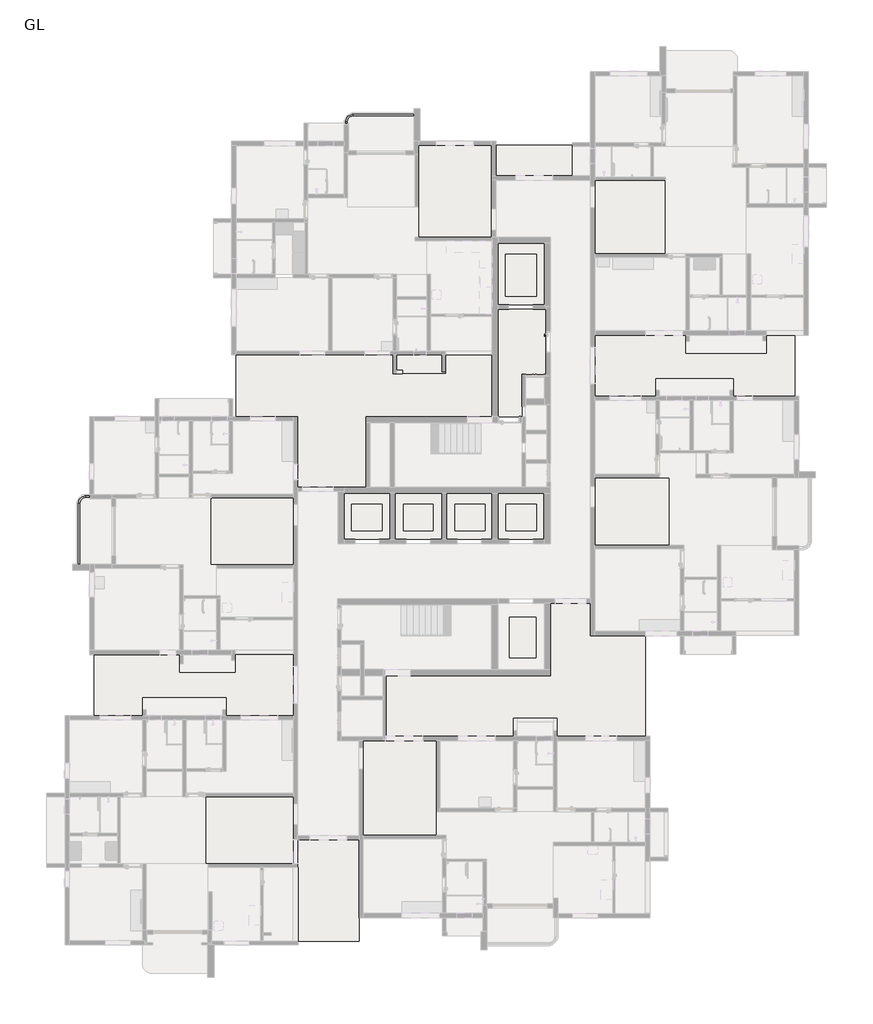
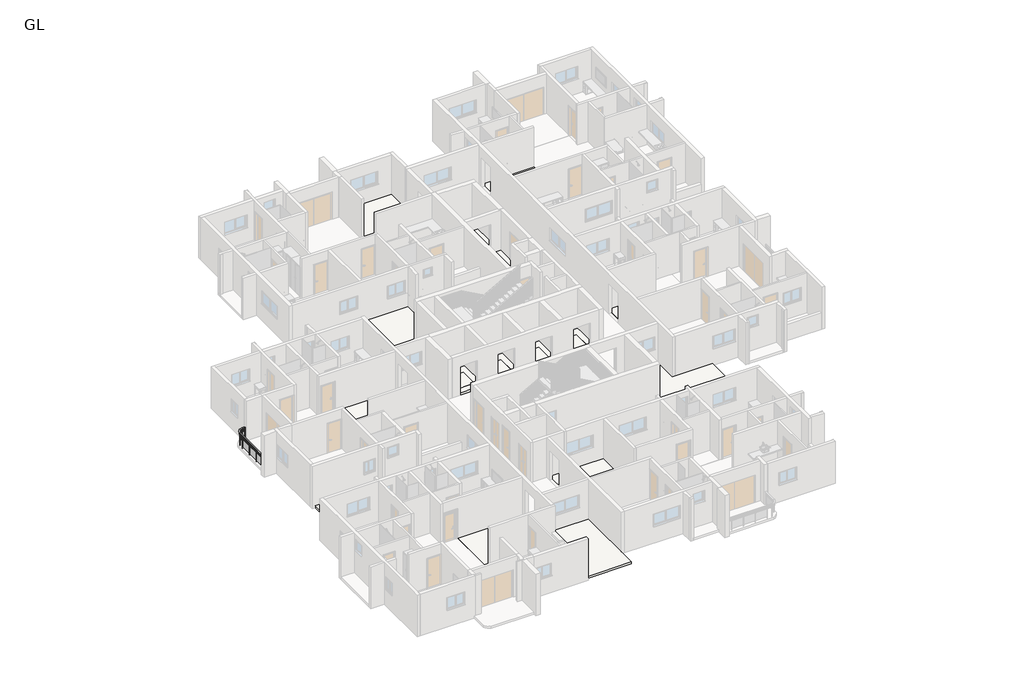
# One storey, part 8 of 14: 6 slabs, 2 railings.
"""IFC4 building model written with IfcOpenShell, lengths in millimetres."""

from ifc_helpers import new_model, si_unit, point, frame, origin, origin_with_axes, place, context, project, spatial, polyline, circle_curve, ellipse_curve, trimmed, outline, extrude, element, save
from ifc_brep_helpers import plane_surface, cylinder_surface, revolved_surface, extruded_surface, advanced_brep

model = new_model("IFC4")

# Units and contexts
model_context = context("Model", 3, world=origin())
ifc_project = project(units=[si_unit("LENGTHUNIT", "METRE", prefix="MILLI")], contexts=[model_context])

# Site, building, storey
site = spatial("IfcSite", under=ifc_project)
building = spatial("IfcBuilding", under=site)
storey = spatial("IfcBuildingStorey", under=building, Name="GL", Elevation=0.0)

# Railings
placement = place(None, origin())
element("IfcRailing", 1, ObjectType="Glass_Panel-Bottom_Fill", at=placement, inside=storey, context=model_context, shape_type="SolidModel", body=[
    advanced_brep(
    [(501.9833716, 97457.1229135, 1049.9616), (501.9833716, 97537.1229135, 1049.9616), (-2551.6680428, 97457.1229135, 1049.9616), (-2551.6680428, 97537.1229135, 1049.9616), (-2919.9542338, 97168.8367225, 1049.9616), (-2839.9542338, 97168.8367225, 1049.9616), (-2839.9542338, 97086.2867225, 1049.9616), (-2919.9542338, 97086.2867225, 1049.9616)],
    [
        (0, 1, ellipse_curve(frame((501.9833716, 97497.1229135, 1049.9616), z_axis=(1.0, 0.0, 0.0), x_axis=(0.0, 1.0, 0.0)), 40.0, 30.0)),
        (1, 0, ellipse_curve(frame((501.9833716, 97497.1229135, 1049.9616), z_axis=(1.0, 0.0, 0.0), x_axis=(0.0, 1.0, 0.0)), 40.0, 30.0)),
        (0, 2),
        (2, 3, ellipse_curve(frame((-2551.6680428, 97497.1229135, 1049.9616), z_axis=(1.0, 0.0, 0.0), x_axis=(0.0, 1.0, 0.0)), 40.0, 30.0)),
        (3, 1),
        (3, 2, ellipse_curve(frame((-2551.6680428, 97497.1229135, 1049.9616), z_axis=(1.0, 0.0, 0.0), x_axis=(0.0, 1.0, 0.0)), 40.0, 30.0)),
        (4, 3, circle_curve(frame((-2551.6680428, 97168.8367225, 1049.9616), z_axis=(0.0, 0.0, -1.0), x_axis=(0.0, 1.0, 0.0)), 368.286191)),
        (2, 5, circle_curve(frame((-2551.6680428, 97168.8367225, 1049.9616), z_axis=(0.0, 0.0, 1.0), x_axis=(0.0, 1.0, 0.0)), 288.286191)),
        (5, 4, ellipse_curve(frame((-2879.9542338, 97168.8367225, 1049.9616), z_axis=(0.0, 1.0, 0.0), x_axis=(-1.0, 0.0, 0.0)), 40.0, 30.0)),
        (4, 5, ellipse_curve(frame((-2879.9542338, 97168.8367225, 1049.9616), z_axis=(0.0, 1.0, 0.0), x_axis=(-1.0, 0.0, 0.0)), 40.0, 30.0)),
        (6, 7, ellipse_curve(frame((-2879.9542338, 97086.2867225, 1049.9616), z_axis=(0.0, -1.0, 0.0), x_axis=(-1.0, 0.0, 0.0)), 40.0, 30.0)),
        (7, 6, ellipse_curve(frame((-2879.9542338, 97086.2867225, 1049.9616), z_axis=(0.0, -1.0, 0.0), x_axis=(-1.0, 0.0, 0.0)), 40.0, 30.0)),
        (5, 6),
        (7, 4),
    ],
    [
        plane_surface(frame((501.9833716, 97497.1229135, 1049.9616), z_axis=(1.0, 0.0, 0.0), x_axis=(0.0, -1.0, 0.0))),
        extruded_surface(trimmed(ellipse_curve(frame((-2551.6680428, 97497.1229135, 1049.9616), z_axis=(1.0, 0.0, 0.0), x_axis=(0.0, 1.0, 0.0)), 40.0, 30.0), [point((-2551.6680428, 97457.1229135, 1049.9616))], [point((-2551.6680428, 97537.1229135, 1049.9616))], True, "CARTESIAN"), (3053.6514144, 0.0, 0.0), 3053.6514144),
        extruded_surface(trimmed(ellipse_curve(frame((-2551.6680428, 97497.1229135, 1049.9616), z_axis=(1.0, 0.0, 0.0), x_axis=(0.0, 1.0, 0.0)), 40.0, 30.0), [point((-2551.6680428, 97537.1229135, 1049.9616))], [point((-2551.6680428, 97457.1229135, 1049.9616))], True, "CARTESIAN"), (3053.6514144, 0.0, 0.0), 3053.6514144),
        revolved_surface(trimmed(ellipse_curve(frame((-2551.6680428, 97497.1229135, 1049.9616), z_axis=(1.0, 0.0, 0.0), x_axis=(0.0, 1.0, 0.0)), 40.0, 30.0), [point((-2551.6680428, 97457.1229135, 1049.9616))], [point((-2551.6680428, 97537.1229135, 1049.9616))], True, "CARTESIAN"), (-2551.6680428, 97168.8367225, 1049.9616), (0.0, 0.0, 1.0)),
        revolved_surface(trimmed(ellipse_curve(frame((-2551.6680428, 97497.1229135, 1049.9616), z_axis=(1.0, 0.0, 0.0), x_axis=(0.0, 1.0, 0.0)), 40.0, 30.0), [point((-2551.6680428, 97537.1229135, 1049.9616))], [point((-2551.6680428, 97457.1229135, 1049.9616))], True, "CARTESIAN"), (-2551.6680428, 97168.8367225, 1049.9616), (0.0, 0.0, 1.0)),
        plane_surface(frame((-2879.9542338, 97086.2867225, 1049.9616), z_axis=(0.0, -1.0, 0.0), x_axis=(0.0, 0.0, -1.0))),
        extruded_surface(trimmed(ellipse_curve(frame((-2879.9542338, 97086.2867225, 1049.9616), z_axis=(0.0, 1.0, 0.0), x_axis=(-1.0, 0.0, 0.0)), 40.0, 30.0), [point((-2839.9542338, 97086.2867225, 1049.9616))], [point((-2919.9542338, 97086.2867225, 1049.9616))], True, "CARTESIAN"), (0.0, 82.55000000000291, 0.0), 82.55000000000291),
        extruded_surface(trimmed(ellipse_curve(frame((-2879.9542338, 97086.2867225, 1049.9616), z_axis=(0.0, 1.0, 0.0), x_axis=(-1.0, 0.0, 0.0)), 40.0, 30.0), [point((-2919.9542338, 97086.2867225, 1049.9616))], [point((-2839.9542338, 97086.2867225, 1049.9616))], True, "CARTESIAN"), (0.0, 82.55000000000291, 0.0), 82.55000000000291),
    ],
    [
        (0, [[1, 2]]),
        (1, [[-1, 3, 4, 5]]),
        (2, [[-2, -5, 6, -3]]),
        (3, [[7, -4, 8, 9]]),
        (4, [[-8, -6, -7, 10]]),
        (5, [[11, 12]]),
        (6, [[-9, 13, -12, 14]]),
        (7, [[-10, -14, -11, -13]]),
    ],
),
    advanced_brep(
    [(501.9833716, 97506.5136787, 949.9616), (501.9833716, 97486.5136787, 949.9616), (501.9833716, 97486.5136787, 929.9616), (501.9833716, 97506.5136787, 929.9616), (-2551.6680428, 97506.5136787, 949.9616), (-2551.6680428, 97486.5136787, 949.9616), (-2551.6680428, 97486.5136787, 929.9616), (-2551.6680428, 97506.5136787, 929.9616), (-2869.344999, 97168.8367225, 949.9616), (-2889.344999, 97168.8367225, 949.9616), (-2869.344999, 97168.8367225, 929.9616), (-2889.344999, 97168.8367225, 929.9616), (-2889.344999, 97086.2867225, 949.9616), (-2889.344999, 97086.2867225, 929.9616), (-2869.344999, 97086.2867225, 929.9616), (-2869.344999, 97086.2867225, 949.9616)],
    [
        (0, 1),
        (1, 2),
        (2, 3),
        (3, 0),
        (0, 4),
        (4, 5),
        (5, 1),
        (5, 6),
        (6, 2),
        (6, 7),
        (7, 3),
        (7, 4),
        (8, 5, circle_curve(frame((-2551.6680428, 97168.8367225, 949.9616), z_axis=(0.0, 0.0, -1.0), x_axis=(0.0, 1.0, 0.0)), 317.6769562)),
        (4, 9, circle_curve(frame((-2551.6680428, 97168.8367225, 949.9616), z_axis=(0.0, 0.0, 1.0), x_axis=(0.0, 1.0, 0.0)), 337.6769562)),
        (9, 8),
        (10, 6, circle_curve(frame((-2551.6680428, 97168.8367225, 929.9616), z_axis=(0.0, 0.0, -1.0), x_axis=(0.0, 1.0, 0.0)), 317.6769562)),
        (8, 10),
        (11, 7, circle_curve(frame((-2551.6680428, 97168.8367225, 929.9616), z_axis=(0.0, 0.0, -1.0), x_axis=(0.0, 1.0, 0.0)), 337.6769562)),
        (10, 11),
        (11, 9),
        (12, 13),
        (13, 14),
        (14, 15),
        (15, 12),
        (9, 12),
        (15, 8),
        (14, 10),
        (13, 11),
    ],
    [
        plane_surface(frame((501.9833716, 97496.5136787, 949.9616), z_axis=(1.0, 0.0, 0.0), x_axis=(0.0, -1.0, 0.0))),
        plane_surface(frame((501.9833716, 97506.5136787, 949.9616), z_axis=(0.0, 0.0, 1.0), x_axis=(-1.0, 0.0, 0.0))),
        plane_surface(frame((501.9833716, 97486.5136787, 949.9616), z_axis=(0.0, -1.0, 0.0), x_axis=(-1.0, 0.0, 0.0))),
        plane_surface(frame((501.9833716, 97486.5136787, 929.9616), z_axis=(0.0, 0.0, -1.0), x_axis=(-1.0, 0.0, 0.0))),
        plane_surface(frame((501.9833716, 97506.5136787, 929.9616), z_axis=(0.0, 1.0, 0.0), x_axis=(-1.0, 0.0, 0.0))),
        plane_surface(frame((-2551.6680428, 97168.8367225, 949.9616), z_axis=(0.0, 0.0, 1.0), x_axis=(0.0, 1.0, 0.0))),
        revolved_surface(polyline([(-2551.6680428, 97486.5136787, 949.9616), (-2551.6680428, 97486.5136787, 929.9616)]), (-2551.6680428, 97168.8367225, 949.9616), (0.0, 0.0, 1.0)),
        plane_surface(frame((-2551.6680428, 97168.8367225, 929.9616), z_axis=(0.0, 0.0, -1.0), x_axis=(0.0, 1.0, 0.0))),
        cylinder_surface(frame((-2551.6680428, 97168.8367225, 949.9616), z_axis=(0.0, 0.0, 1.0), x_axis=(0.0, 1.0, 0.0)), 337.6769562),
        plane_surface(frame((-2879.344999, 97086.2867225, 949.9616), z_axis=(0.0, -1.0, 0.0), x_axis=(0.0, 0.0, -1.0))),
        plane_surface(frame((-2889.344999, 97168.8367225, 949.9616), z_axis=(0.0, 0.0, 1.0), x_axis=(0.0, -1.0, 0.0))),
        plane_surface(frame((-2869.344999, 97168.8367225, 949.9616), z_axis=(1.0, 0.0, 0.0), x_axis=(0.0, -1.0, 0.0))),
        plane_surface(frame((-2869.344999, 97168.8367225, 929.9616), z_axis=(0.0, 0.0, -1.0), x_axis=(0.0, -1.0, 0.0))),
        plane_surface(frame((-2889.344999, 97168.8367225, 929.9616), z_axis=(-1.0, 0.0, 0.0), x_axis=(0.0, -1.0, 0.0))),
    ],
    [
        (0, [[1, 2, 3, 4]]),
        (1, [[-1, 5, 6, 7]]),
        (2, [[-2, -7, 8, 9]]),
        (3, [[-3, -9, 10, 11]]),
        (4, [[-4, -11, 12, -5]]),
        (5, [[13, -6, 14, 15]]),
        (6, [[16, -8, -13, 17]]),
        (7, [[18, -10, -16, 19]]),
        (8, [[-14, -12, -18, 20]]),
        (9, [[21, 22, 23, 24]]),
        (10, [[-15, 25, -24, 26]]),
        (11, [[-17, -26, -23, 27]]),
        (12, [[-19, -27, -22, 28]]),
        (13, [[-20, -28, -21, -25]]),
    ],
),
    advanced_brep(
    [(501.9833716, 97506.5136787, 849.9616), (501.9833716, 97486.5136787, 849.9616), (501.9833716, 97486.5136787, 829.9616), (501.9833716, 97506.5136787, 829.9616), (-2551.6680428, 97506.5136787, 849.9616), (-2551.6680428, 97486.5136787, 849.9616), (-2551.6680428, 97486.5136787, 829.9616), (-2551.6680428, 97506.5136787, 829.9616), (-2869.344999, 97168.8367225, 849.9616), (-2889.344999, 97168.8367225, 849.9616), (-2869.344999, 97168.8367225, 829.9616), (-2889.344999, 97168.8367225, 829.9616), (-2889.344999, 97086.2867225, 849.9616), (-2889.344999, 97086.2867225, 829.9616), (-2869.344999, 97086.2867225, 829.9616), (-2869.344999, 97086.2867225, 849.9616)],
    [
        (0, 1),
        (1, 2),
        (2, 3),
        (3, 0),
        (0, 4),
        (4, 5),
        (5, 1),
        (5, 6),
        (6, 2),
        (6, 7),
        (7, 3),
        (7, 4),
        (8, 5, circle_curve(frame((-2551.6680428, 97168.8367225, 849.9616), z_axis=(0.0, 0.0, -1.0), x_axis=(0.0, 1.0, 0.0)), 317.6769562)),
        (4, 9, circle_curve(frame((-2551.6680428, 97168.8367225, 849.9616), z_axis=(0.0, 0.0, 1.0), x_axis=(0.0, 1.0, 0.0)), 337.6769562)),
        (9, 8),
        (10, 6, circle_curve(frame((-2551.6680428, 97168.8367225, 829.9616), z_axis=(0.0, 0.0, -1.0), x_axis=(0.0, 1.0, 0.0)), 317.6769562)),
        (8, 10),
        (11, 7, circle_curve(frame((-2551.6680428, 97168.8367225, 829.9616), z_axis=(0.0, 0.0, -1.0), x_axis=(0.0, 1.0, 0.0)), 337.6769562)),
        (10, 11),
        (11, 9),
        (12, 13),
        (13, 14),
        (14, 15),
        (15, 12),
        (9, 12),
        (15, 8),
        (14, 10),
        (13, 11),
    ],
    [
        plane_surface(frame((501.9833716, 97496.5136787, 849.9616), z_axis=(1.0, 0.0, 0.0), x_axis=(0.0, -1.0, 0.0))),
        plane_surface(frame((501.9833716, 97506.5136787, 849.9616), z_axis=(0.0, 0.0, 1.0), x_axis=(-1.0, 0.0, 0.0))),
        plane_surface(frame((501.9833716, 97486.5136787, 849.9616), z_axis=(0.0, -1.0, 0.0), x_axis=(-1.0, 0.0, 0.0))),
        plane_surface(frame((501.9833716, 97486.5136787, 829.9616), z_axis=(0.0, 0.0, -1.0), x_axis=(-1.0, 0.0, 0.0))),
        plane_surface(frame((501.9833716, 97506.5136787, 829.9616), z_axis=(0.0, 1.0, 0.0), x_axis=(-1.0, 0.0, 0.0))),
        plane_surface(frame((-2551.6680428, 97168.8367225, 849.9616), z_axis=(0.0, 0.0, 1.0), x_axis=(0.0, 1.0, 0.0))),
        revolved_surface(polyline([(-2551.6680428, 97486.5136787, 849.9616), (-2551.6680428, 97486.5136787, 829.9616)]), (-2551.6680428, 97168.8367225, 849.9616), (0.0, 0.0, 1.0)),
        plane_surface(frame((-2551.6680428, 97168.8367225, 829.9616), z_axis=(0.0, 0.0, -1.0), x_axis=(0.0, 1.0, 0.0))),
        cylinder_surface(frame((-2551.6680428, 97168.8367225, 849.9616), z_axis=(0.0, 0.0, 1.0), x_axis=(0.0, 1.0, 0.0)), 337.6769562),
        plane_surface(frame((-2879.344999, 97086.2867225, 849.9616), z_axis=(0.0, -1.0, 0.0), x_axis=(0.0, 0.0, -1.0))),
        plane_surface(frame((-2889.344999, 97168.8367225, 849.9616), z_axis=(0.0, 0.0, 1.0), x_axis=(0.0, -1.0, 0.0))),
        plane_surface(frame((-2869.344999, 97168.8367225, 849.9616), z_axis=(1.0, 0.0, 0.0), x_axis=(0.0, -1.0, 0.0))),
        plane_surface(frame((-2869.344999, 97168.8367225, 829.9616), z_axis=(0.0, 0.0, -1.0), x_axis=(0.0, -1.0, 0.0))),
        plane_surface(frame((-2889.344999, 97168.8367225, 829.9616), z_axis=(-1.0, 0.0, 0.0), x_axis=(0.0, -1.0, 0.0))),
    ],
    [
        (0, [[1, 2, 3, 4]]),
        (1, [[-1, 5, 6, 7]]),
        (2, [[-2, -7, 8, 9]]),
        (3, [[-3, -9, 10, 11]]),
        (4, [[-4, -11, 12, -5]]),
        (5, [[13, -6, 14, 15]]),
        (6, [[16, -8, -13, 17]]),
        (7, [[18, -10, -16, 19]]),
        (8, [[-14, -12, -18, 20]]),
        (9, [[21, 22, 23, 24]]),
        (10, [[-15, 25, -24, 26]]),
        (11, [[-17, -26, -23, 27]]),
        (12, [[-19, -27, -22, 28]]),
        (13, [[-20, -28, -21, -25]]),
    ],
),
    extrude(outline(polyline([(-2218.8423356, 97471.5136787), (-2230.8423356, 97471.5136787), (-2230.8423356, 97521.5136787), (-2218.8423356, 97521.5136787), (-2218.8423356, 97471.5136787)])), frame((0.0, 0.0, 149.9616), z_axis=(0.0, 0.0, 1.0), x_axis=(1.0, 0.0, 0.0)), (0.0, 0.0, 1.0), 870.0),
    extrude(outline(polyline([(-1424.8423356, 97498.2384888), (-2224.8423356, 97498.2384888), (-2224.8423356, 97503.2384888), (-1424.8423356, 97503.2384888), (-1424.8423356, 97498.2384888)])), frame((0.0, 0.0, 249.9616), z_axis=(0.0, 0.0, 1.0), x_axis=(1.0, 0.0, 0.0)), (0.0, 0.0, 1.0), 580.0),
    extrude(outline(polyline([(-1418.8423356, 97471.5136787), (-1430.8423356, 97471.5136787), (-1430.8423356, 97521.5136787), (-1418.8423356, 97521.5136787), (-1418.8423356, 97471.5136787)])), frame((0.0, 0.0, 149.9616), z_axis=(0.0, 0.0, 1.0), x_axis=(1.0, 0.0, 0.0)), (0.0, 0.0, 1.0), 870.0),
    extrude(outline(polyline([(-624.8423356, 97498.2384888), (-1424.8423356, 97498.2384888), (-1424.8423356, 97503.2384888), (-624.8423356, 97503.2384888), (-624.8423356, 97498.2384888)])), frame((0.0, 0.0, 249.9616), z_axis=(0.0, 0.0, 1.0), x_axis=(1.0, 0.0, 0.0)), (0.0, 0.0, 1.0), 580.0),
    extrude(outline(polyline([(-618.8423356, 97471.5136787), (-630.8423356, 97471.5136787), (-630.8423356, 97521.5136787), (-618.8423356, 97521.5136787), (-618.8423356, 97471.5136787)])), frame((0.0, 0.0, 149.9616), z_axis=(0.0, 0.0, 1.0), x_axis=(1.0, 0.0, 0.0)), (0.0, 0.0, 1.0), 870.0),
    extrude(outline(polyline([(175.1576644, 97498.2384888), (-624.8423356, 97498.2384888), (-624.8423356, 97503.2384888), (175.1576644, 97503.2384888), (175.1576644, 97498.2384888)])), frame((0.0, 0.0, 249.9616), z_axis=(0.0, 0.0, 1.0), x_axis=(1.0, 0.0, 0.0)), (0.0, 0.0, 1.0), 580.0),
    extrude(outline(polyline([(181.1576644, 97471.5136787), (169.1576644, 97471.5136787), (169.1576644, 97521.5136787), (181.1576644, 97521.5136787), (181.1576644, 97471.5136787)])), frame((0.0, 0.0, 149.9616), z_axis=(0.0, 0.0, 1.0), x_axis=(1.0, 0.0, 0.0)), (0.0, 0.0, 1.0), 870.0),
    extrude(outline(polyline([(-2854.344999, 97174.8367225), (-2854.344999, 97162.8367225), (-2904.344999, 97162.8367225), (-2904.344999, 97174.8367225), (-2854.344999, 97174.8367225)])), frame((0.0, 0.0, 149.9616), z_axis=(0.0, 0.0, 1.0), x_axis=(1.0, 0.0, 0.0)), (0.0, 0.0, 1.0), 870.0),
    extrude(outline(polyline([(-2545.6680428, 97471.5136787), (-2557.6680428, 97471.5136787), (-2557.6680428, 97521.5136787), (-2545.6680428, 97521.5136787), (-2545.6680428, 97471.5136787)])), frame((0.0, 0.0, 149.9616), z_axis=(0.0, 0.0, 1.0), x_axis=(1.0, 0.0, 0.0)), (0.0, 0.0, 1.0), 870.0),
    extrude(outline(polyline([(-2854.344999, 97094.2867225), (-2854.344999, 97082.2867225), (-2904.344999, 97082.2867225), (-2904.344999, 97094.2867225), (-2854.344999, 97094.2867225)])), frame((0.0, 0.0, 149.9616), z_axis=(0.0, 0.0, 1.0), x_axis=(1.0, 0.0, 0.0)), (0.0, 0.0, 1.0), 870.0),
    extrude(outline(polyline([(505.9833716, 97471.5136787), (493.9833716, 97471.5136787), (493.9833716, 97521.5136787), (505.9833716, 97521.5136787), (505.9833716, 97471.5136787)])), frame((0.0, 0.0, 149.9616), z_axis=(0.0, 0.0, 1.0), x_axis=(1.0, 0.0, 0.0)), (0.0, 0.0, 1.0), 870.0),
])
element("IfcRailing", 2, ObjectType="Glass_Panel-Bottom_Fill", at=placement, inside=storey, context=model_context, shape_type="SolidModel", body=[
    advanced_brep(
    [(-16238.3038997, 75105.5827724, 1049.9616), (-16158.3038997, 75105.5827724, 1049.9616), (-16238.3038997, 78153.5827724, 1049.9616), (-16158.3038997, 78153.5827724, 1049.9616), (-15865.7412071, 78446.145465, 1049.9616), (-15865.7412071, 78526.145465, 1049.9616), (-15656.6231346, 78526.145465, 1049.9616), (-15656.6231346, 78446.145465, 1049.9616)],
    [
        (0, 1, ellipse_curve(frame((-16198.3038997, 75105.5827724, 1049.9616), z_axis=(0.0, -1.0, 0.0), x_axis=(1.0, 0.0, 0.0)), 40.0, 30.0)),
        (1, 0, ellipse_curve(frame((-16198.3038997, 75105.5827724, 1049.9616), z_axis=(0.0, -1.0, 0.0), x_axis=(1.0, 0.0, 0.0)), 40.0, 30.0)),
        (0, 2),
        (2, 3, ellipse_curve(frame((-16198.3038997, 78153.5827724, 1049.9616), z_axis=(0.0, -1.0, 0.0), x_axis=(1.0, 0.0, 0.0)), 40.0, 30.0)),
        (3, 1),
        (3, 2, ellipse_curve(frame((-16198.3038997, 78153.5827724, 1049.9616), z_axis=(0.0, -1.0, 0.0), x_axis=(1.0, 0.0, 0.0)), 40.0, 30.0)),
        (4, 3, circle_curve(frame((-15865.7412071, 78153.5827724, 1049.9616), z_axis=(0.0, 0.0, 1.0), x_axis=(-1.0, 0.0, 0.0)), 292.5626927)),
        (2, 5, circle_curve(frame((-15865.7412071, 78153.5827724, 1049.9616), z_axis=(0.0, 0.0, -1.0), x_axis=(-1.0, 0.0, 0.0)), 372.5626927)),
        (5, 4, ellipse_curve(frame((-15865.7412071, 78486.145465, 1049.9616), z_axis=(-1.0, 0.0, 0.0), x_axis=(0.0, -1.0, 0.0)), 40.0, 30.0)),
        (4, 5, ellipse_curve(frame((-15865.7412071, 78486.145465, 1049.9616), z_axis=(-1.0, 0.0, 0.0), x_axis=(0.0, -1.0, 0.0)), 40.0, 30.0)),
        (6, 7, ellipse_curve(frame((-15656.6231346, 78486.145465, 1049.9616), z_axis=(1.0, 0.0, 0.0), x_axis=(0.0, -1.0, 0.0)), 40.0, 30.0)),
        (7, 6, ellipse_curve(frame((-15656.6231346, 78486.145465, 1049.9616), z_axis=(1.0, 0.0, 0.0), x_axis=(0.0, -1.0, 0.0)), 40.0, 30.0)),
        (5, 6),
        (7, 4),
    ],
    [
        plane_surface(frame((-16198.3038997, 75105.5827724, 1049.9616), z_axis=(0.0, -1.0, 0.0), x_axis=(0.0, 0.0, 1.0))),
        extruded_surface(trimmed(ellipse_curve(frame((-16198.3038997, 78153.5827724, 1049.9616), z_axis=(0.0, -1.0, 0.0), x_axis=(1.0, 0.0, 0.0)), 40.0, 30.0), [point((-16238.3038997, 78153.5827724, 1049.9616))], [point((-16158.3038997, 78153.5827724, 1049.9616))], True, "CARTESIAN"), (0.0, -3048.0, 0.0), 3048.0),
        extruded_surface(trimmed(ellipse_curve(frame((-16198.3038997, 78153.5827724, 1049.9616), z_axis=(0.0, -1.0, 0.0), x_axis=(1.0, 0.0, 0.0)), 40.0, 30.0), [point((-16158.3038997, 78153.5827724, 1049.9616))], [point((-16238.3038997, 78153.5827724, 1049.9616))], True, "CARTESIAN"), (0.0, -3048.0, 0.0), 3048.0),
        revolved_surface(trimmed(ellipse_curve(frame((-16198.3038997, 78153.5827724, 1049.9616), z_axis=(0.0, -1.0, 0.0), x_axis=(1.0, 0.0, 0.0)), 40.0, 30.0), [point((-16238.3038997, 78153.5827724, 1049.9616))], [point((-16158.3038997, 78153.5827724, 1049.9616))], True, "CARTESIAN"), (-15865.7412071, 78153.5827724, 1049.9616), (0.0, 0.0, -1.0)),
        revolved_surface(trimmed(ellipse_curve(frame((-16198.3038997, 78153.5827724, 1049.9616), z_axis=(0.0, -1.0, 0.0), x_axis=(1.0, 0.0, 0.0)), 40.0, 30.0), [point((-16158.3038997, 78153.5827724, 1049.9616))], [point((-16238.3038997, 78153.5827724, 1049.9616))], True, "CARTESIAN"), (-15865.7412071, 78153.5827724, 1049.9616), (0.0, 0.0, -1.0)),
        plane_surface(frame((-15656.6231346, 78486.145465, 1049.9616), z_axis=(1.0, 0.0, 0.0), x_axis=(0.0, 1.0, 0.0))),
        extruded_surface(trimmed(ellipse_curve(frame((-15656.6231346, 78486.145465, 1049.9616), z_axis=(-1.0, 0.0, 0.0), x_axis=(0.0, -1.0, 0.0)), 40.0, 30.0), [point((-15656.6231346, 78526.145465, 1049.9616))], [point((-15656.6231346, 78446.145465, 1049.9616))], True, "CARTESIAN"), (-209.11807249999947, 0.0, 0.0), 209.11807249999947),
        extruded_surface(trimmed(ellipse_curve(frame((-15656.6231346, 78486.145465, 1049.9616), z_axis=(-1.0, 0.0, 0.0), x_axis=(0.0, -1.0, 0.0)), 40.0, 30.0), [point((-15656.6231346, 78446.145465, 1049.9616))], [point((-15656.6231346, 78526.145465, 1049.9616))], True, "CARTESIAN"), (-209.11807249999947, 0.0, 0.0), 209.11807249999947),
    ],
    [
        (0, [[1, 2]]),
        (1, [[-1, 3, 4, 5]]),
        (2, [[-2, -5, 6, -3]]),
        (3, [[7, -4, 8, 9]]),
        (4, [[-8, -6, -7, 10]]),
        (5, [[11, 12]]),
        (6, [[-9, 13, -12, 14]]),
        (7, [[-10, -14, -11, -13]]),
    ],
),
    advanced_brep(
    [(-16188.9131346, 75105.5827724, 949.9616), (-16208.9131346, 75105.5827724, 949.9616), (-16208.9131346, 75105.5827724, 929.9616), (-16188.9131346, 75105.5827724, 929.9616), (-16188.9131346, 78153.5827724, 949.9616), (-16208.9131346, 78153.5827724, 949.9616), (-16208.9131346, 78153.5827724, 929.9616), (-16188.9131346, 78153.5827724, 929.9616), (-15865.7412071, 78496.7546999, 949.9616), (-15865.7412071, 78476.7546999, 949.9616), (-15865.7412071, 78496.7546999, 929.9616), (-15865.7412071, 78476.7546999, 929.9616), (-15656.6231346, 78476.7546999, 949.9616), (-15656.6231346, 78476.7546999, 929.9616), (-15656.6231346, 78496.7546999, 929.9616), (-15656.6231346, 78496.7546999, 949.9616)],
    [
        (0, 1),
        (1, 2),
        (2, 3),
        (3, 0),
        (0, 4),
        (4, 5),
        (5, 1),
        (5, 6),
        (6, 2),
        (6, 7),
        (7, 3),
        (7, 4),
        (8, 5, circle_curve(frame((-15865.7412071, 78153.5827724, 949.9616), z_axis=(0.0, 0.0, 1.0), x_axis=(-1.0, 0.0, 0.0)), 343.1719275)),
        (4, 9, circle_curve(frame((-15865.7412071, 78153.5827724, 949.9616), z_axis=(0.0, 0.0, -1.0), x_axis=(-1.0, 0.0, 0.0)), 323.1719275)),
        (9, 8),
        (10, 6, circle_curve(frame((-15865.7412071, 78153.5827724, 929.9616), z_axis=(0.0, 0.0, 1.0), x_axis=(-1.0, 0.0, 0.0)), 343.1719275)),
        (8, 10),
        (11, 7, circle_curve(frame((-15865.7412071, 78153.5827724, 929.9616), z_axis=(0.0, 0.0, 1.0), x_axis=(-1.0, 0.0, 0.0)), 323.1719275)),
        (10, 11),
        (11, 9),
        (12, 13),
        (13, 14),
        (14, 15),
        (15, 12),
        (9, 12),
        (15, 8),
        (14, 10),
        (13, 11),
    ],
    [
        plane_surface(frame((-16198.9131346, 75105.5827724, 949.9616), z_axis=(0.0, -1.0, 0.0), x_axis=(0.0, 0.0, 1.0))),
        plane_surface(frame((-16188.9131346, 75105.5827724, 949.9616), z_axis=(0.0, 0.0, 1.0), x_axis=(0.0, 1.0, 0.0))),
        plane_surface(frame((-16208.9131346, 75105.5827724, 949.9616), z_axis=(-1.0, 0.0, 0.0), x_axis=(0.0, 1.0, 0.0))),
        plane_surface(frame((-16208.9131346, 75105.5827724, 929.9616), z_axis=(0.0, 0.0, -1.0), x_axis=(0.0, 1.0, 0.0))),
        plane_surface(frame((-16188.9131346, 75105.5827724, 929.9616), z_axis=(1.0, 0.0, 0.0), x_axis=(0.0, 1.0, 0.0))),
        plane_surface(frame((-15865.7412071, 78153.5827724, 949.9616), z_axis=(0.0, 0.0, 1.0), x_axis=(-1.0, 0.0, 0.0))),
        cylinder_surface(frame((-15865.7412071, 78153.5827724, 949.9616), z_axis=(0.0, 0.0, -1.0), x_axis=(-1.0, 0.0, 0.0)), 343.1719275),
        plane_surface(frame((-15865.7412071, 78153.5827724, 929.9616), z_axis=(0.0, 0.0, -1.0), x_axis=(-1.0, 0.0, 0.0))),
        revolved_surface(polyline([(-16188.9131346, 78153.5827724, 929.9616), (-16188.9131346, 78153.5827724, 949.9616)]), (-15865.7412071, 78153.5827724, 949.9616), (0.0, 0.0, -1.0)),
        plane_surface(frame((-15656.6231346, 78486.7546999, 949.9616), z_axis=(1.0, 0.0, 0.0), x_axis=(0.0, 1.0, 0.0))),
        plane_surface(frame((-15865.7412071, 78476.7546999, 949.9616), z_axis=(0.0, 0.0, 1.0), x_axis=(1.0, 0.0, 0.0))),
        plane_surface(frame((-15865.7412071, 78496.7546999, 949.9616), z_axis=(0.0, 1.0, 0.0), x_axis=(1.0, 0.0, 0.0))),
        plane_surface(frame((-15865.7412071, 78496.7546999, 929.9616), z_axis=(0.0, 0.0, -1.0), x_axis=(1.0, 0.0, 0.0))),
        plane_surface(frame((-15865.7412071, 78476.7546999, 929.9616), z_axis=(0.0, -1.0, 0.0), x_axis=(1.0, 0.0, 0.0))),
    ],
    [
        (0, [[1, 2, 3, 4]]),
        (1, [[-1, 5, 6, 7]]),
        (2, [[-2, -7, 8, 9]]),
        (3, [[-3, -9, 10, 11]]),
        (4, [[-4, -11, 12, -5]]),
        (5, [[13, -6, 14, 15]]),
        (6, [[16, -8, -13, 17]]),
        (7, [[18, -10, -16, 19]]),
        (8, [[-14, -12, -18, 20]]),
        (9, [[21, 22, 23, 24]]),
        (10, [[-15, 25, -24, 26]]),
        (11, [[-17, -26, -23, 27]]),
        (12, [[-19, -27, -22, 28]]),
        (13, [[-20, -28, -21, -25]]),
    ],
),
    advanced_brep(
    [(-16188.9131346, 75105.5827724, 849.9616), (-16208.9131346, 75105.5827724, 849.9616), (-16208.9131346, 75105.5827724, 829.9616), (-16188.9131346, 75105.5827724, 829.9616), (-16188.9131346, 78153.5827724, 849.9616), (-16208.9131346, 78153.5827724, 849.9616), (-16208.9131346, 78153.5827724, 829.9616), (-16188.9131346, 78153.5827724, 829.9616), (-15865.7412071, 78496.7546999, 849.9616), (-15865.7412071, 78476.7546999, 849.9616), (-15865.7412071, 78496.7546999, 829.9616), (-15865.7412071, 78476.7546999, 829.9616), (-15656.6231346, 78476.7546999, 849.9616), (-15656.6231346, 78476.7546999, 829.9616), (-15656.6231346, 78496.7546999, 829.9616), (-15656.6231346, 78496.7546999, 849.9616)],
    [
        (0, 1),
        (1, 2),
        (2, 3),
        (3, 0),
        (0, 4),
        (4, 5),
        (5, 1),
        (5, 6),
        (6, 2),
        (6, 7),
        (7, 3),
        (7, 4),
        (8, 5, circle_curve(frame((-15865.7412071, 78153.5827724, 849.9616), z_axis=(0.0, 0.0, 1.0), x_axis=(-1.0, 0.0, 0.0)), 343.1719275)),
        (4, 9, circle_curve(frame((-15865.7412071, 78153.5827724, 849.9616), z_axis=(0.0, 0.0, -1.0), x_axis=(-1.0, 0.0, 0.0)), 323.1719275)),
        (9, 8),
        (10, 6, circle_curve(frame((-15865.7412071, 78153.5827724, 829.9616), z_axis=(0.0, 0.0, 1.0), x_axis=(-1.0, 0.0, 0.0)), 343.1719275)),
        (8, 10),
        (11, 7, circle_curve(frame((-15865.7412071, 78153.5827724, 829.9616), z_axis=(0.0, 0.0, 1.0), x_axis=(-1.0, 0.0, 0.0)), 323.1719275)),
        (10, 11),
        (11, 9),
        (12, 13),
        (13, 14),
        (14, 15),
        (15, 12),
        (9, 12),
        (15, 8),
        (14, 10),
        (13, 11),
    ],
    [
        plane_surface(frame((-16198.9131346, 75105.5827724, 849.9616), z_axis=(0.0, -1.0, 0.0), x_axis=(0.0, 0.0, 1.0))),
        plane_surface(frame((-16188.9131346, 75105.5827724, 849.9616), z_axis=(0.0, 0.0, 1.0), x_axis=(0.0, 1.0, 0.0))),
        plane_surface(frame((-16208.9131346, 75105.5827724, 849.9616), z_axis=(-1.0, 0.0, 0.0), x_axis=(0.0, 1.0, 0.0))),
        plane_surface(frame((-16208.9131346, 75105.5827724, 829.9616), z_axis=(0.0, 0.0, -1.0), x_axis=(0.0, 1.0, 0.0))),
        plane_surface(frame((-16188.9131346, 75105.5827724, 829.9616), z_axis=(1.0, 0.0, 0.0), x_axis=(0.0, 1.0, 0.0))),
        plane_surface(frame((-15865.7412071, 78153.5827724, 849.9616), z_axis=(0.0, 0.0, 1.0), x_axis=(-1.0, 0.0, 0.0))),
        cylinder_surface(frame((-15865.7412071, 78153.5827724, 849.9616), z_axis=(0.0, 0.0, -1.0), x_axis=(-1.0, 0.0, 0.0)), 343.1719275),
        plane_surface(frame((-15865.7412071, 78153.5827724, 829.9616), z_axis=(0.0, 0.0, -1.0), x_axis=(-1.0, 0.0, 0.0))),
        revolved_surface(polyline([(-16188.9131346, 78153.5827724, 829.9616), (-16188.9131346, 78153.5827724, 849.9616)]), (-15865.7412071, 78153.5827724, 849.9616), (0.0, 0.0, -1.0)),
        plane_surface(frame((-15656.6231346, 78486.7546999, 849.9616), z_axis=(1.0, 0.0, 0.0), x_axis=(0.0, 1.0, 0.0))),
        plane_surface(frame((-15865.7412071, 78476.7546999, 849.9616), z_axis=(0.0, 0.0, 1.0), x_axis=(1.0, 0.0, 0.0))),
        plane_surface(frame((-15865.7412071, 78496.7546999, 849.9616), z_axis=(0.0, 1.0, 0.0), x_axis=(1.0, 0.0, 0.0))),
        plane_surface(frame((-15865.7412071, 78496.7546999, 829.9616), z_axis=(0.0, 0.0, -1.0), x_axis=(1.0, 0.0, 0.0))),
        plane_surface(frame((-15865.7412071, 78476.7546999, 829.9616), z_axis=(0.0, -1.0, 0.0), x_axis=(1.0, 0.0, 0.0))),
    ],
    [
        (0, [[1, 2, 3, 4]]),
        (1, [[-1, 5, 6, 7]]),
        (2, [[-2, -7, 8, 9]]),
        (3, [[-3, -9, 10, 11]]),
        (4, [[-4, -11, 12, -5]]),
        (5, [[13, -6, 14, 15]]),
        (6, [[16, -8, -13, 17]]),
        (7, [[18, -10, -16, 19]]),
        (8, [[-14, -12, -18, 20]]),
        (9, [[21, 22, 23, 24]]),
        (10, [[-15, 25, -24, 26]]),
        (11, [[-17, -26, -23, 27]]),
        (12, [[-19, -27, -22, 28]]),
        (13, [[-20, -28, -21, -25]]),
    ],
),
    extrude(outline(polyline([(-16223.9131346, 77823.5827724), (-16223.9131346, 77835.5827724), (-16173.9131346, 77835.5827724), (-16173.9131346, 77823.5827724), (-16223.9131346, 77823.5827724)])), frame((0.0, 0.0, 149.9616), z_axis=(0.0, 0.0, 1.0), x_axis=(1.0, 0.0, 0.0)), (0.0, 0.0, 1.0), 870.0),
    extrude(outline(polyline([(-16197.1883245, 77029.5827724), (-16197.1883245, 77829.5827724), (-16192.1883245, 77829.5827724), (-16192.1883245, 77029.5827724), (-16197.1883245, 77029.5827724)])), frame((0.0, 0.0, 249.9616), z_axis=(0.0, 0.0, 1.0), x_axis=(1.0, 0.0, 0.0)), (0.0, 0.0, 1.0), 580.0),
    extrude(outline(polyline([(-16223.9131346, 77023.5827724), (-16223.9131346, 77035.5827724), (-16173.9131346, 77035.5827724), (-16173.9131346, 77023.5827724), (-16223.9131346, 77023.5827724)])), frame((0.0, 0.0, 149.9616), z_axis=(0.0, 0.0, 1.0), x_axis=(1.0, 0.0, 0.0)), (0.0, 0.0, 1.0), 870.0),
    extrude(outline(polyline([(-16197.1883245, 76229.5827724), (-16197.1883245, 77029.5827724), (-16192.1883245, 77029.5827724), (-16192.1883245, 76229.5827724), (-16197.1883245, 76229.5827724)])), frame((0.0, 0.0, 249.9616), z_axis=(0.0, 0.0, 1.0), x_axis=(1.0, 0.0, 0.0)), (0.0, 0.0, 1.0), 580.0),
    extrude(outline(polyline([(-16223.9131346, 76223.5827724), (-16223.9131346, 76235.5827724), (-16173.9131346, 76235.5827724), (-16173.9131346, 76223.5827724), (-16223.9131346, 76223.5827724)])), frame((0.0, 0.0, 149.9616), z_axis=(0.0, 0.0, 1.0), x_axis=(1.0, 0.0, 0.0)), (0.0, 0.0, 1.0), 870.0),
    extrude(outline(polyline([(-16197.1883245, 75429.5827724), (-16197.1883245, 76229.5827724), (-16192.1883245, 76229.5827724), (-16192.1883245, 75429.5827724), (-16197.1883245, 75429.5827724)])), frame((0.0, 0.0, 249.9616), z_axis=(0.0, 0.0, 1.0), x_axis=(1.0, 0.0, 0.0)), (0.0, 0.0, 1.0), 580.0),
    extrude(outline(polyline([(-16223.9131346, 75423.5827724), (-16223.9131346, 75435.5827724), (-16173.9131346, 75435.5827724), (-16173.9131346, 75423.5827724), (-16223.9131346, 75423.5827724)])), frame((0.0, 0.0, 149.9616), z_axis=(0.0, 0.0, 1.0), x_axis=(1.0, 0.0, 0.0)), (0.0, 0.0, 1.0), 870.0),
    extrude(outline(polyline([(-15871.7412071, 78511.7546999), (-15859.7412071, 78511.7546999), (-15859.7412071, 78461.7546999), (-15871.7412071, 78461.7546999), (-15871.7412071, 78511.7546999)])), frame((0.0, 0.0, 149.9616), z_axis=(0.0, 0.0, 1.0), x_axis=(1.0, 0.0, 0.0)), (0.0, 0.0, 1.0), 870.0),
    extrude(outline(polyline([(-16223.9131346, 78147.5827724), (-16223.9131346, 78159.5827724), (-16173.9131346, 78159.5827724), (-16173.9131346, 78147.5827724), (-16223.9131346, 78147.5827724)])), frame((0.0, 0.0, 149.9616), z_axis=(0.0, 0.0, 1.0), x_axis=(1.0, 0.0, 0.0)), (0.0, 0.0, 1.0), 870.0),
    extrude(outline(polyline([(-15664.6231346, 78511.7546999), (-15652.6231346, 78511.7546999), (-15652.6231346, 78461.7546999), (-15664.6231346, 78461.7546999), (-15664.6231346, 78511.7546999)])), frame((0.0, 0.0, 149.9616), z_axis=(0.0, 0.0, 1.0), x_axis=(1.0, 0.0, 0.0)), (0.0, 0.0, 1.0), 870.0),
    extrude(outline(polyline([(-16223.9131346, 75101.5827724), (-16223.9131346, 75113.5827724), (-16173.9131346, 75113.5827724), (-16173.9131346, 75101.5827724), (-16223.9131346, 75101.5827724)])), frame((0.0, 0.0, 149.9616), z_axis=(0.0, 0.0, 1.0), x_axis=(1.0, 0.0, 0.0)), (0.0, 0.0, 1.0), 870.0),
])

# Slabs
element("IfcSlab", 3, ObjectType="DRAWING FLOORING", at=placement, inside=storey, context=model_context, shape_type="SweptSolid", body=[
    extrude(outline(polyline([(13025.3335039, 94229.5349831), (13025.3335039, 90571.6728694), (9508.1569726, 90571.6728694), (9508.1569726, 94229.5349831), (13025.3335039, 94229.5349831)])), origin_with_axes(), (0.0, 0.0, 1.0), 149.9616),
    extrude(outline(polyline([(13222.0624579, 79413.1078957), (13222.0624579, 76055.2491416), (9508.1569726, 76055.2491416), (9508.1569726, 79413.1078957), (13222.0624579, 79413.1078957)])), origin_with_axes(), (0.0, 0.0, 1.0), 149.9616),
    extrude(outline(polyline([(1620.577694, 66313.8928421), (1620.577694, 61604.2127724), (-2044.3665436, 61604.2127724), (-2044.3665436, 66313.8928421), (1620.577694, 66313.8928421)])), origin_with_axes(), (0.0, 0.0, 1.0), 149.9616),
    extrude(outline(polyline([(-9878.7762852, 60152.7487724), (-9878.7762852, 63501.9127724), (-5517.8131346, 63501.9127724), (-5517.8131346, 60152.7487724), (-9878.7762852, 60152.7487724)])), origin_with_axes(), (0.0, 0.0, 1.0), 149.9616),
    extrude(outline(polyline([(-9633.0131346, 75074.8487724), (-9633.0131346, 78399.0127724), (-5492.8131346, 78399.0127724), (-5492.8131346, 75074.8487724), (-9633.0131346, 75074.8487724)])), origin_with_axes(), (0.0, 0.0, 1.0), 149.9616),
    extrude(outline(polyline([(715.3433716, 91396.9573985), (715.3433716, 95980.6109831), (4369.7369726, 95980.6109831), (4369.7369726, 91396.9573985), (715.3433716, 91396.9573985)])), origin_with_axes(), (0.0, 0.0, 1.0), 149.9616),
])
element("IfcSlab", 4, ObjectType="LIFT FLOORING 1", at=placement, inside=storey, context=model_context, shape_type="SweptSolid", body=[
    extrude(outline(polyline([(-686.4678446, 78643.5487724), (-686.4678446, 76353.9927724), (-2983.2931346, 76353.9927724), (-2983.2931346, 78643.5487724), (-686.4678446, 78643.5487724)]), holes=[polyline([(-1088.5269558, 78097.0898759), (-2612.5269558, 78097.0898759), (-2612.5269558, 76776.2898759), (-1088.5269558, 76776.2898759), (-1088.5269558, 78097.0898759)])]), origin_with_axes(), (0.0, 0.0, 1.0), 149.9616),
    extrude(outline(polyline([(1881.4721554, 78643.5487724), (1881.4721554, 76353.9927724), (-442.6278446, 76353.9927724), (-442.6278446, 78643.5487724), (1881.4721554, 78643.5487724)]), holes=[polyline([(1456.9364295, 78097.0898759), (-23.5193089, 78097.0898759), (-23.5193089, 76776.2898759), (1456.9364295, 76776.2898759), (1456.9364295, 78097.0898759)])]), origin_with_axes(), (0.0, 0.0, 1.0), 149.9616),
    extrude(outline(polyline([(4382.7068654, 78643.5487724), (4382.7068654, 76353.9927724), (2125.3121554, 76353.9927724), (2125.3121554, 78643.5487724), (4382.7068654, 78643.5487724)]), holes=[polyline([(4033.5766081, 78097.0898759), (2536.9410256, 78097.0898759), (2536.9410256, 76776.2898759), (4033.5766081, 76776.2898759), (4033.5766081, 78097.0898759)])]), origin_with_axes(), (0.0, 0.0, 1.0), 149.9616),
    extrude(outline(polyline([(6986.2068654, 78643.5487724), (6986.2068654, 76353.9927724), (4687.5068654, 76353.9927724), (4687.5068654, 78643.5487724), (6986.2068654, 78643.5487724)]), holes=[polyline([(6594.0369426, 78097.0898759), (5081.2215159, 78097.0898759), (5081.2215159, 76776.2898759), (6594.0369426, 76776.2898759), (6594.0369426, 78097.0898759)])]), origin_with_axes(), (0.0, 0.0, 1.0), 149.9616),
    extrude(outline(polyline([(6993.0368387, 91092.1573985), (6993.0368387, 88039.0502935), (4681.6368387, 88039.0502935), (4681.6368387, 91092.1573985), (6993.0368387, 91092.1573985)]), holes=[polyline([(6608.2803831, 90551.6039668), (5058.8803831, 90551.6039668), (5058.8803831, 88468.8039668), (6608.2803831, 88468.8039668), (6608.2803831, 90551.6039668)])]), origin_with_axes(), (0.0, 0.0, 1.0), 149.9616),
])
element("IfcSlab", 5, ObjectType="LIFT FLOORING 2", at=placement, inside=storey, context=model_context, shape_type="SweptSolid", body=[
    extrude(outline(polyline([(-1088.5269558, 78097.0898759), (-1088.5269558, 76776.2898759), (-2612.5269558, 76776.2898759), (-2612.5269558, 78097.0898759), (-1088.5269558, 78097.0898759)])), origin_with_axes(), (0.0, 0.0, 1.0), 149.9616),
    extrude(outline(polyline([(1456.9364295, 78097.0898759), (1456.9364295, 76776.2898759), (-23.5193089, 76776.2898759), (-23.5193089, 78097.0898759), (1456.9364295, 78097.0898759)])), origin_with_axes(), (0.0, 0.0, 1.0), 149.9616),
    extrude(outline(polyline([(4033.5766081, 78097.0898759), (4033.5766081, 76776.2898759), (2536.9410256, 76776.2898759), (2536.9410256, 78097.0898759), (4033.5766081, 78097.0898759)])), origin_with_axes(), (0.0, 0.0, 1.0), 149.9616),
    extrude(outline(polyline([(6594.0369426, 78097.0898759), (6594.0369426, 76776.2898759), (5081.2215159, 76776.2898759), (5081.2215159, 78097.0898759), (6594.0369426, 78097.0898759)])), origin_with_axes(), (0.0, 0.0, 1.0), 149.9616),
    extrude(outline(polyline([(6608.2803831, 90551.6039668), (6608.2803831, 88468.8039668), (5058.8803831, 88468.8039668), (5058.8803831, 90551.6039668), (6608.2803831, 90551.6039668)])), origin_with_axes(), (0.0, 0.0, 1.0), 149.9616),
    extrude(outline(polyline([(6566.7895687, 72477.0600946), (6566.7895687, 70445.0600946), (5245.9895687, 70445.0600946), (5245.9895687, 72477.0600946), (6566.7895687, 72477.0600946)])), origin_with_axes(), (0.0, 0.0, 1.0), 149.9616),
])
element("IfcSlab", 6, ObjectType="LOBBY", at=placement, inside=storey, context=model_context, shape_type="SweptSolid", body=[
    extrude(outline(polyline([(7068.7568654, 87816.5462935), (7068.7568654, 84574.4487724), (5874.9568654, 84574.4487724), (5874.9568654, 82462.5073985), (4681.6368387, 82462.5073985), (4681.6368387, 87816.5462935), (7068.7568654, 87816.5462935)])), origin_with_axes(), (0.0, 0.0, 1.0), 149.9616),
])
element("IfcSlab", 7, ObjectType="OUTDOOR FLOORING", at=placement, inside=storey, context=model_context, shape_type="SweptSolid", body=[
    extrude(outline(polyline([(4376.8368387, 85548.0073985), (4376.8368387, 82462.5073985), (-1903.3131613, 82462.5073985), (-1903.3131613, 78948.3487724), (-5294.6931346, 78948.3487724), (-5294.6931346, 82463.1246999), (-8373.9631613, 82463.1246999), (-8373.9631613, 85522.6073985), (-550.7631613, 85522.6073985), (-550.7631613, 84608.2073985), (2090.8368387, 84608.2073985), (2090.8368387, 85548.0073985), (4376.8368387, 85548.0073985)])), origin_with_axes(), (0.0, 0.0, 1.0), 149.9616),
    extrude(outline(polyline([(14061.4115488, 86531.4578957), (14061.4115488, 85629.02324), (18054.9396703, 85629.02324), (18054.9396703, 86531.4578957), (19477.3396703, 86531.4578957), (19477.3396703, 83487.2678957), (16405.6984579, 83487.2678957), (16405.6984579, 84364.6781404), (12563.4404579, 84364.6781404), (12563.4404579, 83487.2678957), (9508.1569726, 83487.2678957), (9508.1569726, 86531.4578957), (14061.4115488, 86531.4578957)])), origin_with_axes(), (0.0, 0.0, 1.0), 149.9616),
    extrude(outline(polyline([(8391.2620982, 95980.6109831), (8391.2620982, 94454.0709831), (4583.0969726, 94454.0709831), (4583.0969726, 95980.6109831), (8391.2620982, 95980.6109831)])), origin_with_axes(), (0.0, 0.0, 1.0), 149.9616),
    extrude(outline(polyline([(-2242.4865436, 61393.3927724), (-2242.4865436, 56341.0496151), (-5276.2431346, 56341.0496151), (-5276.2431346, 61393.3927724), (-2242.4865436, 61393.3927724)])), origin_with_axes(), (0.0, 0.0, 1.0), 149.9616),
    extrude(outline(polyline([(-5492.8131346, 67565.5934152), (-8857.9146601, 67565.5934152), (-8857.9146601, 68468.5387344), (-13038.2100711, 68468.5387344), (-13038.2100711, 67565.5934152), (-15452.1531346, 67565.5934152), (-15452.1531346, 70609.7827724), (-11178.6031346, 70609.7827724), (-11178.6031346, 69729.9714811), (-8413.8131346, 69729.9714811), (-8413.8131346, 70609.7827724), (-5492.8131346, 70609.7827724), (-5492.8131346, 67565.5934152)])), origin_with_axes(), (0.0, 0.0, 1.0), 149.9616),
    extrude(outline(polyline([(7306.113694, 69561.3033979), (7306.113694, 73177.9138911), (9294.7969726, 73177.9138911), (9294.7969726, 71549.2678957), (12037.9969726, 71549.2678957), (12037.9969726, 66531.0628421), (7623.613694, 66531.0628421), (7623.613694, 67430.8578421), (5455.977694, 67430.8578421), (5455.977694, 66531.0628421), (-885.386306, 66531.0628421), (-885.386306, 69561.3033979), (7306.113694, 69561.3033979)])), origin_with_axes(), (0.0, 0.0, 1.0), 149.9616),
])
element("IfcSlab", 8, ObjectType="SHAFT", at=placement, inside=storey, context=model_context, shape_type="SweptSolid", body=[
    extrude(outline(polyline([(2073.655001, 85538.1556254), (2073.655001, 84611.0556254), (-538.480999, 84611.0556254), (-538.480999, 85538.1556254), (2073.655001, 85538.1556254)])), origin_with_axes(), (0.0, 0.0, 1.0), 149.9616),
])

save(model, "model.ifc")

# Revit data of these elements
# Type "Glass_Panel-Bottom_Fill"
#   built-in parameter 1008612 = 0.019685 (stored number, unit not read)
#   built-in parameter 1008611 = 0.019685 (stored number, unit not read)
#   built-in parameter 1008609 = 0.902231 (stored number, unit not read)
#   built-in parameter 1008604 = 0.19685 (stored number, unit not read)
#   built-in parameter 1008603 = 0.164042 (stored number, unit not read)
#   Railing Height = 2.952756 ft
#   built-in parameter 1008630 = 2
#   built-in parameter 1008610 = 2
# Type "DRAWING FLOORING"
#   Function = 0
#   Layers, outside or top first: 0.072 ft "HALL" (function 5); 0.42 ft "Structure, Timber Joist/Rafter Layer" (function 1)
# Type "LIFT FLOORING 1"
#   Function = 0
#   Layers, outside or top first: 0.072 ft "LIFT OUT" (function 5); 0.42 ft "Structure, Timber Joist/Rafter Layer" (function 1)
# Type "LIFT FLOORING 2"
#   Function = 0
#   Layers, outside or top first: 0.072 ft "LIFT IN" (function 5); 0.42 ft "Structure, Timber Joist/Rafter Layer" (function 1)
# Type "LOBBY"
#   Function = 0
#   Layers, outside or top first: 0.072 ft "LOBBY" (function 5); 0.42 ft "Structure, Timber Joist/Rafter Layer" (function 1)
# Type "OUTDOOR FLOORING"
#   Function = 0
#   Layers, outside or top first: 0.072 ft "OUTDOOR FLOORING" (function 5); 0.42 ft "Structure, Timber Joist/Rafter Layer" (function 1)
# Type "SHAFT"
#   Function = 0
#   Layers, outside or top first: 0.072 ft "SHAFT" (function 5); 0.42 ft "Structure, Timber Joist/Rafter Layer" (function 1)
# Elements 1, 2 (IfcRailing, "Glass_Panel-Bottom_Fill")
#   built-in parameter 1008621 = 0.492 (stored number, unit not read)
#   Phase Created = New Construction
#   Materials on its faces: "Metal - Stainless Steel,Polished", "Glass"
# Element 3 (IfcSlab, "DRAWING FLOORING")
#   Height Offset From Level = 0.492 ft
#   Phase Created = New Construction
#   Materials on its faces: "Structure, Timber Joist/Rafter Layer", "HALL"
# Element 4 (IfcSlab, "LIFT FLOORING 1")
#   Height Offset From Level = 0.492 ft
#   Phase Created = New Construction
#   Materials on its faces: "Structure, Timber Joist/Rafter Layer", "LIFT OUT"
# Element 5 (IfcSlab, "LIFT FLOORING 2")
#   Height Offset From Level = 0.492 ft
#   Phase Created = New Construction
#   Materials on its faces: "Structure, Timber Joist/Rafter Layer", "LIFT IN"
# Element 6 (IfcSlab, "LOBBY")
#   Height Offset From Level = 0.492 ft
#   Phase Created = New Construction
#   Materials on its faces: "Structure, Timber Joist/Rafter Layer", "LOBBY"
# Element 7 (IfcSlab, "OUTDOOR FLOORING")
#   built-in parameter 1001955 = 1.5708 (stored number, unit not read)
#   Height Offset From Level = 0.492 ft
#   Phase Created = New Construction
#   Materials on its faces: "Structure, Timber Joist/Rafter Layer", "OUTDOOR FLOORING"
# Element 8 (IfcSlab, "SHAFT")
#   Height Offset From Level = 0.492 ft
#   Phase Created = New Construction
#   Materials on its faces: "Structure, Timber Joist/Rafter Layer", "SHAFT"
# Materials
#   "HALL": class "Generic", colour RGB 120 120 120, transparency 0, Cost = 0
#   "Structure, Timber Joist/Rafter Layer": class "Wood", colour RGB 127 127 127, transparency 0, Description = "Timber framing, thermal airspace", Cost = 0
#   "LIFT OUT": class "Generic", colour RGB 120 120 120, transparency 0, Cost = 0
#   "LIFT IN": class "Generic", colour RGB 120 120 120, transparency 0, Cost = 0
#   "LOBBY": class "Generic", colour RGB 120 120 120, transparency 0, Cost = 0
#   "OUTDOOR FLOORING": class "Generic", colour RGB 120 120 120, transparency 0, Cost = 0
#   "SHAFT": class "Generic", colour RGB 120 120 120, transparency 0, Cost = 0
#   "Metal - Stainless Steel,Polished": class "Metal", colour RGB 236 239 239, transparency 0, Cost = 0
#   "Glass": class "Glass", colour RGB 0 128 192, transparency 0.9, Description = "Soda Lime Glass", Cost = 0
